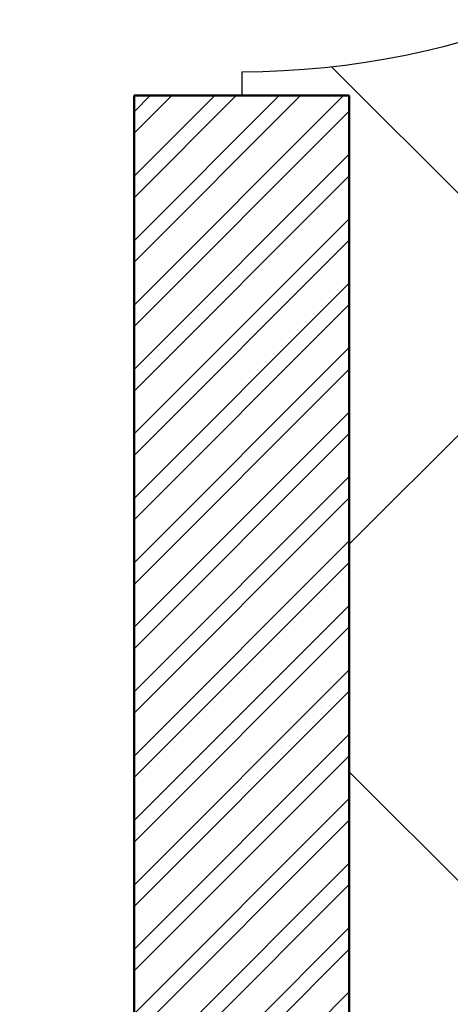
# Model space of a CAD drawing. Units: inches. Extents: x 3590 to 5167, y 65 to 1917.
# Tile 64 of 100: x 4919 to 4937, y 1681 to 1722. Entities that reach past the tile are written whole.
import ezdxf

# ---------------------------------------------------------------- set-up
doc = ezdxf.new("R2010")
doc.units = ezdxf.units.IN
for name, color, linetype, lineweight in [('A-DOOR', 3, 'Continuous', 25), ('A-FLOR-PATT', 8, 'Continuous', 13), ('A-WALL', 7, 'Continuous', 50), ('A-WALL-PATT', 251, 'Continuous', 13)]:
    doc.layers.add(name, color=color, linetype=linetype, lineweight=lineweight)

# ---------------------------------------------------------------- blocks, each defined once
blk = doc.blocks.new('D1')
for p, q in [((1, 0), (1, 34)), ((2, 0), (2, 33.985)), ((0, 0), (2, 0)), ((35, 0), (36, 0))]:
    blk.add_line(p, q)
at = {"ltscale": 0.5}
blk.add_arc((1, 0), 34, 0, 90, dxfattribs=at)

msp = doc.modelspace()

# ---------------------------------------------------------------- hatches: boundary and pattern name
at = {"layer": 'A-FLOR-PATT', "transparency": 33554687}
h = msp.add_hatch(dxfattribs=at)
h.set_pattern_fill('AR-HBONE', color=256, scale=0.2)
h.set_pattern_definition([(45, (-588.972, 0), (0, 28.73682), [60.96, -20.32]), (135, (-574.604, 14.368), (3e-15, 28.73682), [60.96, -20.32])])
h.paths.add_polyline_path([(5071.274, 1796.999), (4933.274, 1796.999), (4933.274, 1753.999), (4962.774, 1753.999, -0.414214), (4928.774, 1719.999), (4933.274, 1718.999), (4933.274, 1334.999), (5071.274, 1334.999)])
h.paths.add_polyline_path([(4951.78, 1521.077), (4951.715, 1521.04), (4951.563, 1520.895)], flags=16)
h.paths.add_polyline_path([(4952.267, 1521.376), (4952.198, 1521.371), (4952.198, 1521.356)], flags=0)
h.paths.add_polyline_path([(4967.051, 1529.728), (4965.231, 1528.694), (4963.411, 1527.714), (4961.756, 1526.851), (4963.589, 1527.449), (4964.036, 1527.478), (4962.975, 1527.249), (4961.76, 1526.852), (4959.792, 1525.834), (4958.005, 1524.895), (4956.24, 1523.93), (4954.504, 1522.919), (4954.129, 1522.682), (4953.361, 1521.997), (4953.366, 1521.998), (4953.605, 1522.064), (4955.106, 1522.761), (4956.921, 1523.434), (4958.678, 1523.915), (4960.358, 1524.2), (4961.945, 1524.286), (4964.171, 1524.108), (4965.958, 1523.309), (4963.863, 1522.976), (4965.187, 1522.499), (4963.366, 1522.497), (4961.545, 1522.487), (4959.764, 1522.461), (4958.304, 1522.419), (4957.974, 1522.388), (4956.307, 1522.232), (4954.718, 1522.071), (4953.251, 1521.899), (4953.525, 1521.623), (4954.331, 1521.379), (4956.243, 1521.23), (4958.039, 1520.93), (4959.684, 1520.483), (4961.16, 1519.896), (4963.107, 1518.8), (4964.393, 1517.325), (4962.973, 1517.726), (4964.558, 1516.661), (4965.407, 1515.708), (4963.507, 1516.322), (4961.68, 1517.005), (4959.935, 1517.745), (4958.282, 1518.528), (4956.732, 1519.343), (4955.295, 1520.175), (4954.672, 1520.572), (4954.513, 1520.627), (4955.658, 1519.318), (4956.703, 1517.982), (4957.644, 1516.647), (4958.485, 1515.334), (4959.55, 1513.524), (4960.438, 1511.769), (4958.841, 1513.62), (4957.452, 1515.325), (4955.819, 1517.459), (4956.665, 1515.448), (4957.111, 1513.923), (4957.447, 1511.714), (4957.076, 1509.793), (4956.538, 1511.11), (4955.992, 1512.569), (4955.444, 1514.125), (4954.898, 1515.735), (4954.357, 1517.356), (4953.824, 1518.943), (4953.305, 1520.452), (4953.065, 1521.116), (4952.971, 1521.146), (4952.949, 1521.086), (4952.73, 1520.199), (4953.37, 1518.024), (4953.757, 1516.373), (4954.051, 1514.765), (4954.264, 1513.221), (4954.471, 1511.131), (4954.497, 1510.402), (4954.409, 1511.76), (4954.264, 1513.221), (4954.051, 1514.765), (4953.757, 1516.373), (4953.37, 1518.024), (4952.877, 1519.698), (4952.716, 1520.141), (4952.533, 1519.059), (4952.374, 1517.789), (4952.219, 1516.312), (4952.046, 1514.6), (4951.833, 1512.626), (4951.557, 1510.363), (4951.203, 1512.168), (4950.852, 1514.339), (4950.985, 1516.376), (4951.66, 1518.286), (4952.593, 1520.481), (4952.357, 1521.13), (4951.855, 1520.328), (4950.839, 1518.908), (4949.777, 1517.587), (4948.916, 1516.617), (4948.111, 1515.256), (4947.089, 1513.554), (4945.889, 1511.615), (4946.326, 1513.402), (4946.562, 1514.249), (4945.528, 1513.327), (4944.581, 1512.531), (4946.018, 1514.508), (4947.204, 1516.048), (4947.893, 1517.313), (4949.307, 1518.764), (4950.414, 1519.767), (4950.451, 1519.806), (4952.267, 1521.376), (4951.645, 1521.493), (4950.404, 1521.18), (4948.044, 1520.359), (4946.119, 1519.452), (4944.572, 1518.475), (4943.35, 1517.443), (4941.997, 1515.92), (4941.661, 1515.275), (4942.813, 1516.99), (4944.572, 1518.475), (4946.119, 1519.452), (4948.044, 1520.359), (4950.404, 1521.18), (4951.645, 1521.493), (4949.647, 1521.868), (4948.6, 1521.756), (4947.126, 1521.57), (4945.42, 1521.348), (4943.45, 1521.105), (4941.183, 1520.856), (4942.86, 1521.613), (4943.873, 1522.03), (4942.952, 1521.909), (4941.41, 1521.485), (4939.543, 1520.67), (4938.968, 1520.226), (4940.733, 1521.299), (4942.952, 1521.909), (4943.702, 1522.008), (4945.894, 1522.7), (4947.565, 1522.714), (4948.921, 1522.566), (4951.131, 1522.183), (4950.971, 1522.297), (4948.129, 1523.006), (4946.035, 1523.707), (4944.232, 1524.521), (4942.707, 1525.461), (4941.444, 1526.537), (4940.43, 1527.761), (4939.649, 1529.143), (4941.421, 1528.122), (4943.147, 1527.132), (4944.841, 1526.175), (4946.514, 1525.25), (4948.179, 1524.359), (4948.365, 1524.263), (4946.475, 1526.045), (4945.181, 1527.54), (4944.19, 1529.033), (4943.496, 1530.54), (4943.278, 1531.36), (4942.498, 1531.919), (4943.114, 1531.762), (4942.959, 1533.659), (4944.14, 1531.989), (4944.612, 1531.323), (4946.202, 1530.463), (4947.486, 1529.509), (4948.79, 1528.226), (4950.368, 1526.237), (4949.485, 1528.155), (4948.851, 1530.123), (4948.491, 1532.041), (4948.381, 1533.918), (4948.501, 1535.76), (4948.827, 1537.573), (4949.418, 1535.565), (4949.957, 1533.569), (4950.464, 1531.586), (4950.961, 1529.617), (4951.391, 1527.954), (4951.724, 1530.687), (4952.201, 1532.58), (4952.889, 1534.33), (4953.77, 1535.951), (4954.827, 1537.46), (4954.521, 1535.39), (4954.273, 1533.937), (4955.58, 1535.663), (4956.748, 1536.739), (4956.159, 1534.78), (4955.589, 1532.873), (4955.043, 1531.006), (4954.525, 1529.166), (4954.038, 1527.341), (4953.638, 1525.733), (4953.611, 1525.586), (4953.398, 1524.166), (4953.382, 1524.009), (4954.07, 1525.476), (4954.912, 1527.022), (4956.136, 1528.894), (4957.847, 1530.577), (4959.376, 1531.54), (4958.256, 1530.104), (4957.143, 1528.663), (4956.066, 1527.243), (4955.056, 1525.871), (4954.141, 1524.571), (4953.352, 1523.372), (4953.311, 1523.303), (4953.273, 1522.925), (4953.261, 1522.382), (4954.103, 1523.373), (4954.63, 1524.284), (4955.961, 1526.358), (4957.23, 1528.13), (4958.421, 1529.609), (4960.037, 1531.368), (4961.374, 1532.375), (4962.101, 1532.77), (4961.07, 1531.061), (4959.987, 1529.438), (4958.869, 1527.908), (4958.15, 1527.007), (4959.803, 1528.003), (4961.589, 1528.793), (4963.391, 1529.328), (4965.211, 1529.632)], flags=16)
h.paths.add_polyline_path([(4962.944, 1523.182), (4961.107, 1523.422), (4960.392, 1523.362), (4962.35, 1523.331)], flags=0)
h.paths.add_polyline_path([(5049.541, 1584.551), (5049.476, 1584.515), (5049.325, 1584.37)], flags=16)
h.paths.add_polyline_path([(5050.028, 1584.851), (5049.959, 1584.845), (5049.959, 1584.83)], flags=0)
h.paths.add_polyline_path([(5042.333, 1581.949), (5043.88, 1582.926), (5045.806, 1583.833), (5048.165, 1584.654), (5049.406, 1584.967), (5047.408, 1585.342), (5046.361, 1585.231), (5044.888, 1585.044), (5043.181, 1584.822), (5041.211, 1584.579), (5038.944, 1584.33), (5040.622, 1585.087), (5041.634, 1585.504), (5040.713, 1585.383), (5039.171, 1584.959), (5037.304, 1584.144), (5036.729, 1583.7), (5038.494, 1584.773), (5040.713, 1585.383), (5041.463, 1585.482), (5043.655, 1586.174), (5045.326, 1586.188), (5046.682, 1586.04), (5048.893, 1585.657), (5048.732, 1585.771), (5045.891, 1586.48), (5043.796, 1587.181), (5041.994, 1587.996), (5040.468, 1588.935), (5039.205, 1590.011), (5038.191, 1591.235), (5037.41, 1592.617), (5039.182, 1591.596), (5040.909, 1590.607), (5042.602, 1589.649), (5044.275, 1588.724), (5045.94, 1587.833), (5046.126, 1587.738), (5044.237, 1589.519), (5042.942, 1591.015), (5041.952, 1592.508), (5041.257, 1594.014), (5041.039, 1594.834), (5040.26, 1595.393), (5040.875, 1595.237), (5040.721, 1597.133), (5041.901, 1595.463), (5042.373, 1594.798), (5043.963, 1593.938), (5045.247, 1592.983), (5046.552, 1591.701), (5048.129, 1589.712), (5047.247, 1591.63), (5046.613, 1593.597), (5046.252, 1595.515), (5046.142, 1597.392), (5046.262, 1599.234), (5046.588, 1601.047), (5047.179, 1599.039), (5047.718, 1597.043), (5048.225, 1595.06), (5048.722, 1593.091), (5049.152, 1591.429), (5049.485, 1594.161), (5049.962, 1596.054), (5050.65, 1597.804), (5051.532, 1599.425), (5052.589, 1600.934), (5052.283, 1598.864), (5052.034, 1597.411), (5053.341, 1599.137), (5054.509, 1600.213), (5053.92, 1598.254), (5053.35, 1596.348), (5052.805, 1594.48), (5052.286, 1592.64), (5051.799, 1590.815), (5051.4, 1589.207), (5051.373, 1589.06), (5051.159, 1587.64), (5051.143, 1587.483), (5051.831, 1588.95), (5052.673, 1590.496), (5053.898, 1592.368), (5055.608, 1594.051), (5057.137, 1595.014), (5056.017, 1593.578), (5054.904, 1592.137), (5053.828, 1590.717), (5052.817, 1589.345), (5051.902, 1588.046), (5051.113, 1586.846), (5051.072, 1586.777), (5051.034, 1586.399), (5051.022, 1585.856), (5051.864, 1586.847), (5052.391, 1587.758), (5053.723, 1589.832), (5054.991, 1591.604), (5056.182, 1593.083), (5057.798, 1594.842), (5059.135, 1595.849), (5059.863, 1596.244), (5058.831, 1594.535), (5057.749, 1592.912), (5056.63, 1591.382), (5055.912, 1590.482), (5057.564, 1591.477), (5059.35, 1592.267), (5061.152, 1592.802), (5062.972, 1593.106), (5064.812, 1593.203), (5062.992, 1592.169), (5061.172, 1591.188), (5059.518, 1590.325), (5061.35, 1590.924), (5061.797, 1590.952), (5060.737, 1590.723), (5059.521, 1590.326), (5057.553, 1589.308), (5055.766, 1588.369), (5054.002, 1587.404), (5052.265, 1586.393), (5051.891, 1586.156), (5051.122, 1585.471), (5051.127, 1585.472), (5051.366, 1585.538), (5052.867, 1586.235), (5054.682, 1586.908), (5056.439, 1587.389), (5058.12, 1587.675), (5059.706, 1587.76), (5061.933, 1587.583), (5063.719, 1586.783), (5061.624, 1586.45), (5062.949, 1585.973), (5061.127, 1585.971), (5059.307, 1585.961), (5057.525, 1585.935), (5056.065, 1585.893), (5055.735, 1585.862), (5054.068, 1585.707), (5052.479, 1585.546), (5051.012, 1585.373), (5051.286, 1585.097), (5052.092, 1584.853), (5054.004, 1584.704), (5055.8, 1584.404), (5057.446, 1583.958), (5058.921, 1583.37), (5060.868, 1582.274), (5062.154, 1580.799), (5060.734, 1581.2), (5062.32, 1580.135), (5063.168, 1579.182), (5061.269, 1579.796), (5059.441, 1580.479), (5057.696, 1581.219), (5056.043, 1582.003), (5054.493, 1582.817), (5053.057, 1583.649), (5052.433, 1584.047), (5052.274, 1584.101), (5053.42, 1582.793), (5054.464, 1581.457), (5055.405, 1580.121), (5056.247, 1578.809), (5057.311, 1576.998), (5058.199, 1575.244), (5056.602, 1577.094), (5055.213, 1578.799), (5053.58, 1580.933), (5054.427, 1578.922), (5054.872, 1577.397), (5055.208, 1575.189), (5054.838, 1573.267), (5054.299, 1574.584), (5053.754, 1576.043), (5053.206, 1577.599), (5052.659, 1579.209), (5052.118, 1580.83), (5051.585, 1582.417), (5051.066, 1583.927), (5050.826, 1584.59), (5050.733, 1584.62), (5050.711, 1584.561), (5050.491, 1583.673), (5051.131, 1581.498), (5051.518, 1579.847), (5051.813, 1578.24), (5052.026, 1576.695), (5052.233, 1574.605), (5052.258, 1573.876), (5052.17, 1575.234), (5052.026, 1576.695), (5051.813, 1578.24), (5051.518, 1579.847), (5051.131, 1581.498), (5050.638, 1583.172), (5050.477, 1583.615), (5050.294, 1582.533), (5050.136, 1581.263), (5049.981, 1579.786), (5049.807, 1578.074), (5049.594, 1576.1), (5049.318, 1573.837), (5048.965, 1575.642), (5048.613, 1577.813), (5048.747, 1579.85), (5049.421, 1581.76), (5050.354, 1583.955), (5050.118, 1584.604), (5049.616, 1583.802), (5048.6, 1582.382), (5047.538, 1581.061), (5046.677, 1580.091), (5045.872, 1578.73), (5044.85, 1577.028), (5043.651, 1575.089), (5044.087, 1576.877), (5044.324, 1577.723), (5043.289, 1576.801), (5042.342, 1576.005), (5043.779, 1577.982), (5044.966, 1579.522), (5045.655, 1580.787), (5047.068, 1582.239), (5048.175, 1583.241), (5048.213, 1583.28), (5050.028, 1584.851), (5049.406, 1584.967), (5048.165, 1584.654), (5045.806, 1583.833), (5043.88, 1582.926), (5042.333, 1581.949), (5041.111, 1580.917), (5039.758, 1579.394), (5039.423, 1578.749), (5040.575, 1580.464)], flags=16)
h.paths.add_polyline_path([(4954.799, 1533.12), (4954.262, 1532.079), (4953.831, 1530.935), (4953.505, 1529.636), (4953.283, 1528.133), (4953.167, 1526.376), (4953.156, 1524.315), (4953.277, 1521.236), (4952.802, 1521.842), (4951.557, 1521.998), (4950.976, 1521.961), (4952.661, 1521.941), (4952.802, 1521.842), (4953.152, 1523.593), (4953.167, 1526.376), (4953.283, 1528.133), (4953.609, 1530.346), (4954.456, 1532.592)], flags=0)
h.paths.add_polyline_path([(5050.563, 1585.316), (5049.318, 1585.472), (5048.737, 1585.435), (5050.422, 1585.415), (5050.563, 1585.316), (5050.914, 1587.067), (5050.928, 1589.851), (5051.045, 1591.607), (5051.371, 1593.82), (5052.217, 1596.066), (5052.56, 1596.594), (5052.024, 1595.554), (5051.592, 1594.409), (5051.266, 1593.11), (5051.045, 1591.607), (5050.928, 1589.851), (5050.918, 1587.789), (5051.038, 1584.71)], flags=0)
h.paths.add_polyline_path([(5058.153, 1586.836), (5060.111, 1586.805), (5060.705, 1586.656), (5058.868, 1586.896)], flags=0)
h.paths.add_polyline_path([(5049.541, 1430.936), (5049.476, 1430.9), (5049.325, 1430.755)], flags=16)
h.paths.add_polyline_path([(5050.028, 1431.236), (5049.959, 1431.231), (5049.959, 1431.215)], flags=0)
h.paths.add_polyline_path([(5046.588, 1447.432), (5047.179, 1445.425), (5047.718, 1443.429), (5048.225, 1441.446), (5048.722, 1439.476), (5049.152, 1437.814), (5049.485, 1440.546), (5049.962, 1442.439), (5050.65, 1444.189), (5051.532, 1445.811), (5052.589, 1447.319), (5052.283, 1445.249), (5052.034, 1443.796), (5053.341, 1445.522), (5054.509, 1446.598), (5053.92, 1444.64), (5053.35, 1442.733), (5052.805, 1440.865), (5052.286, 1439.025), (5051.799, 1437.201), (5051.4, 1435.592), (5051.373, 1435.445), (5051.159, 1434.025), (5051.143, 1433.868), (5051.831, 1435.335), (5052.673, 1436.881), (5053.898, 1438.753), (5055.608, 1440.436), (5057.137, 1441.4), (5056.017, 1439.963), (5054.904, 1438.522), (5053.828, 1437.102), (5052.817, 1435.73), (5051.902, 1434.431), (5051.113, 1433.231), (5051.072, 1433.162), (5051.034, 1432.784), (5051.022, 1432.242), (5051.864, 1433.232), (5052.391, 1434.143), (5053.723, 1436.217), (5054.991, 1437.989), (5056.182, 1439.468), (5057.798, 1441.227), (5059.135, 1442.235), (5059.863, 1442.629), (5058.831, 1440.921), (5057.749, 1439.298), (5056.63, 1437.767), (5055.912, 1436.867), (5057.564, 1437.863), (5059.35, 1438.652), (5061.152, 1439.187), (5062.972, 1439.491), (5064.812, 1439.588), (5062.992, 1438.554), (5061.172, 1437.573), (5059.518, 1436.71), (5061.35, 1437.309), (5061.797, 1437.337), (5060.737, 1437.108), (5059.521, 1436.711), (5057.553, 1435.693), (5055.766, 1434.754), (5054.002, 1433.789), (5052.265, 1432.778), (5051.891, 1432.541), (5051.122, 1431.856), (5051.127, 1431.857), (5051.366, 1431.923), (5052.867, 1432.62), (5054.682, 1433.293), (5056.439, 1433.775), (5058.12, 1434.06), (5059.706, 1434.145), (5061.933, 1433.968), (5063.719, 1433.168), (5061.624, 1432.835), (5062.949, 1432.358), (5061.127, 1432.357), (5059.307, 1432.346), (5057.525, 1432.32), (5056.065, 1432.278), (5055.735, 1432.248), (5054.068, 1432.092), (5052.479, 1431.931), (5051.012, 1431.759), (5051.286, 1431.482), (5052.092, 1431.238), (5054.004, 1431.089), (5055.8, 1430.789), (5057.446, 1430.343), (5058.921, 1429.755), (5060.868, 1428.66), (5062.154, 1427.185), (5060.734, 1427.585), (5062.32, 1426.52), (5063.168, 1425.567), (5061.269, 1426.181), (5059.441, 1426.865), (5057.696, 1427.604), (5056.043, 1428.388), (5054.493, 1429.202), (5053.057, 1430.034), (5052.433, 1430.432), (5052.274, 1430.487), (5053.42, 1429.178), (5054.464, 1427.842), (5055.405, 1426.506), (5056.247, 1425.194), (5057.311, 1423.383), (5058.199, 1421.629), (5056.602, 1423.479), (5055.213, 1425.184), (5053.58, 1427.318), (5054.427, 1425.307), (5054.872, 1423.782), (5055.208, 1421.574), (5054.838, 1419.652), (5054.299, 1420.97), (5053.754, 1422.428), (5053.206, 1423.984), (5052.659, 1425.595), (5052.118, 1427.215), (5051.585, 1428.802), (5051.066, 1430.312), (5050.826, 1430.975), (5050.733, 1431.005), (5050.711, 1430.946), (5050.491, 1430.058), (5051.131, 1427.883), (5051.518, 1426.232), (5051.813, 1424.625), (5052.026, 1423.081), (5052.233, 1420.991), (5052.258, 1420.261), (5052.17, 1421.619), (5052.026, 1423.081), (5051.813, 1424.625), (5051.518, 1426.232), (5051.131, 1427.883), (5050.638, 1429.558), (5050.477, 1430.001), (5050.294, 1428.918), (5050.136, 1427.648), (5049.981, 1426.171), (5049.807, 1424.459), (5049.594, 1422.485), (5049.318, 1420.222), (5048.965, 1422.028), (5048.613, 1424.199), (5048.747, 1426.235), (5049.421, 1428.146), (5050.354, 1430.34), (5050.118, 1430.989), (5049.616, 1430.187), (5048.6, 1428.768), (5047.538, 1427.446), (5046.677, 1426.477), (5045.872, 1425.116), (5044.85, 1423.413), (5043.651, 1421.474), (5044.087, 1423.262), (5044.324, 1424.109), (5043.289, 1423.186), (5042.342, 1422.391), (5043.779, 1424.368), (5044.966, 1425.907), (5045.655, 1427.173), (5047.068, 1428.624), (5048.175, 1429.627), (5048.213, 1429.666), (5050.028, 1431.236), (5049.406, 1431.353), (5048.165, 1431.039), (5045.806, 1430.218), (5043.88, 1429.311), (5042.333, 1428.334), (5041.111, 1427.302), (5039.758, 1425.779), (5039.423, 1425.134), (5040.575, 1426.849), (5042.333, 1428.334), (5043.88, 1429.311), (5045.806, 1430.218), (5048.165, 1431.039), (5049.406, 1431.353), (5047.408, 1431.727), (5046.361, 1431.616), (5044.888, 1431.429), (5043.181, 1431.207), (5041.211, 1430.964), (5038.944, 1430.715), (5040.622, 1431.472), (5041.634, 1431.89), (5040.713, 1431.769), (5039.171, 1431.345), (5037.304, 1430.53), (5036.729, 1430.085), (5038.494, 1431.158), (5040.713, 1431.769), (5041.463, 1431.867), (5043.655, 1432.559), (5045.326, 1432.573), (5046.682, 1432.425), (5048.893, 1432.042), (5048.732, 1432.156), (5045.891, 1432.865), (5043.796, 1433.566), (5041.994, 1434.381), (5040.468, 1435.321), (5039.205, 1436.396), (5038.191, 1437.62), (5037.41, 1439.002), (5039.182, 1437.982), (5040.909, 1436.992), (5042.602, 1436.034), (5044.275, 1435.109), (5045.94, 1434.218), (5046.126, 1434.123), (5044.237, 1435.904), (5042.942, 1437.4), (5041.952, 1438.893), (5041.257, 1440.399), (5041.039, 1441.219), (5040.26, 1441.778), (5040.875, 1441.622), (5040.721, 1443.518), (5041.901, 1441.848), (5042.373, 1441.183), (5043.963, 1440.323), (5045.247, 1439.369), (5046.552, 1438.086), (5048.129, 1436.097), (5047.247, 1438.015), (5046.613, 1439.982), (5046.252, 1441.901), (5046.142, 1443.778), (5046.262, 1445.619)], flags=16)
h.paths.add_polyline_path([(5052.382, 1444.255), (5051.623, 1442.78), (5052.024, 1441.939), (5052.56, 1442.98)], flags=0)
h.paths.add_polyline_path([(5050.563, 1431.701), (5049.318, 1431.857), (5048.737, 1431.821), (5050.422, 1431.8)], flags=0)
h.paths.add_polyline_path([(5058.153, 1433.221), (5060.111, 1433.19), (5060.705, 1433.041), (5058.868, 1433.281)], flags=0)
h.paths.add_polyline_path([(5049.541, 1352.285), (5049.476, 1352.249), (5049.325, 1352.104)], flags=16)
h.paths.add_polyline_path([(5050.028, 1352.585), (5049.959, 1352.58), (5049.959, 1352.564)], flags=0)
h.paths.add_polyline_path([(5046.588, 1368.781), (5047.179, 1366.774), (5047.718, 1364.778), (5048.225, 1362.795), (5048.722, 1360.825), (5049.152, 1359.163), (5049.485, 1361.896), (5049.962, 1363.789), (5050.65, 1365.538), (5051.532, 1367.16), (5052.589, 1368.669), (5052.283, 1366.598), (5052.034, 1365.145), (5053.341, 1366.871), (5054.509, 1367.947), (5053.92, 1365.989), (5053.35, 1364.082), (5052.805, 1362.214), (5052.286, 1360.374), (5051.799, 1358.55), (5051.4, 1356.942), (5051.373, 1356.794), (5051.159, 1355.374), (5051.143, 1355.218), (5051.831, 1356.684), (5052.673, 1358.23), (5053.898, 1360.102), (5055.608, 1361.786), (5057.137, 1362.749), (5056.017, 1361.313), (5054.904, 1359.872), (5053.828, 1358.452), (5052.817, 1357.079), (5051.902, 1355.78), (5051.113, 1354.581), (5051.072, 1354.512), (5051.034, 1354.133), (5051.022, 1353.591), (5051.864, 1354.581), (5052.391, 1355.492), (5053.723, 1357.566), (5054.991, 1359.338), (5056.182, 1360.817), (5057.798, 1362.577), (5059.135, 1363.584), (5059.863, 1363.979), (5058.831, 1362.27), (5057.749, 1360.647), (5056.63, 1359.117), (5055.912, 1358.216), (5057.564, 1359.212), (5059.35, 1360.001), (5061.152, 1360.536), (5062.972, 1360.841), (5064.812, 1360.937), (5062.992, 1359.903), (5061.172, 1358.923), (5059.518, 1358.059), (5061.35, 1358.658), (5061.797, 1358.687), (5060.737, 1358.458), (5059.521, 1358.061), (5057.553, 1357.043), (5055.766, 1356.103), (5054.002, 1355.138), (5052.265, 1354.127), (5051.891, 1353.89), (5051.122, 1353.206), (5051.127, 1353.206), (5051.366, 1353.272), (5052.867, 1353.969), (5054.682, 1354.643), (5056.439, 1355.124), (5058.12, 1355.409), (5059.706, 1355.495), (5061.933, 1355.317), (5063.719, 1354.518), (5061.624, 1354.184), (5062.949, 1353.708), (5061.127, 1353.706), (5059.307, 1353.695), (5057.525, 1353.669), (5056.065, 1353.627), (5055.735, 1353.597), (5054.068, 1353.441), (5052.479, 1353.28), (5051.012, 1353.108), (5051.286, 1352.831), (5052.092, 1352.587), (5054.004, 1352.439), (5055.8, 1352.138), (5057.446, 1351.692), (5058.921, 1351.104), (5060.868, 1350.009), (5062.154, 1348.534), (5060.734, 1348.935), (5062.32, 1347.869), (5063.168, 1346.916), (5061.269, 1347.53), (5059.441, 1348.214), (5057.696, 1348.954), (5056.043, 1349.737), (5054.493, 1350.551), (5053.057, 1351.383), (5052.433, 1351.781), (5052.274, 1351.836), (5053.42, 1350.527), (5054.464, 1349.191), (5055.405, 1347.855), (5056.247, 1346.543), (5057.311, 1344.733), (5058.199, 1342.978), (5056.602, 1344.828), (5055.213, 1346.534), (5053.58, 1348.667), (5054.427, 1346.656), (5054.872, 1345.132), (5055.208, 1342.923), (5054.838, 1341.002), (5054.299, 1342.319), (5053.754, 1343.778), (5053.206, 1345.334), (5052.659, 1346.944), (5052.118, 1348.564), (5051.585, 1350.151), (5051.066, 1351.661), (5050.826, 1352.324), (5050.733, 1352.355), (5050.711, 1352.295), (5050.491, 1351.408), (5051.131, 1349.232), (5051.518, 1347.581), (5051.813, 1345.974), (5052.026, 1344.43), (5052.233, 1342.34), (5052.258, 1341.61), (5052.17, 1342.969), (5052.026, 1344.43), (5051.813, 1345.974), (5051.518, 1347.581), (5051.131, 1349.232), (5050.638, 1350.907), (5050.477, 1351.35), (5050.294, 1350.267), (5050.136, 1348.997), (5049.981, 1347.52), (5049.807, 1345.809), (5049.594, 1343.835), (5049.318, 1341.571), (5048.965, 1343.377), (5048.613, 1345.548), (5048.747, 1347.585), (5049.421, 1349.495), (5050.354, 1351.689), (5050.118, 1352.339), (5049.616, 1351.536), (5048.6, 1350.117), (5047.538, 1348.795), (5046.677, 1347.826), (5045.872, 1346.465), (5044.85, 1344.763), (5043.651, 1342.824), (5044.087, 1344.611), (5044.324, 1345.458), (5043.289, 1344.535), (5042.342, 1343.74), (5043.779, 1345.717), (5044.966, 1347.256), (5045.655, 1348.522), (5047.068, 1349.973), (5048.175, 1350.976), (5048.213, 1351.015), (5050.028, 1352.585), (5049.406, 1352.702), (5048.165, 1352.388), (5045.806, 1351.567), (5043.88, 1350.661), (5042.333, 1349.683), (5041.111, 1348.651), (5039.758, 1347.128), (5039.423, 1346.483), (5040.575, 1348.198), (5042.333, 1349.683), (5043.88, 1350.661), (5045.806, 1351.567), (5048.165, 1352.388), (5049.406, 1352.702), (5047.408, 1353.076), (5046.361, 1352.965), (5044.888, 1352.779), (5043.181, 1352.556), (5041.211, 1352.313), (5038.944, 1352.065), (5040.622, 1352.821), (5041.634, 1353.239), (5040.713, 1353.118), (5039.171, 1352.694), (5037.304, 1351.879), (5036.729, 1351.434), (5038.494, 1352.508), (5040.713, 1353.118), (5041.463, 1353.216), (5043.655, 1353.909), (5045.326, 1353.923), (5046.682, 1353.774), (5048.893, 1353.391), (5048.732, 1353.506), (5045.891, 1354.214), (5043.796, 1354.915), (5041.994, 1355.73), (5040.468, 1356.67), (5039.205, 1357.746), (5038.191, 1358.969), (5037.41, 1360.352), (5039.182, 1359.331), (5040.909, 1358.341), (5042.602, 1357.383), (5044.275, 1356.458), (5045.94, 1355.567), (5046.126, 1355.472), (5044.237, 1357.253), (5042.942, 1358.749), (5041.952, 1360.242), (5041.257, 1361.748), (5041.039, 1362.568), (5040.26, 1363.128), (5040.875, 1362.971), (5040.721, 1364.867), (5041.901, 1363.197), (5042.373, 1362.532), (5043.963, 1361.672), (5045.247, 1360.718), (5046.552, 1359.435), (5048.129, 1357.446), (5047.247, 1359.364), (5046.613, 1361.331), (5046.252, 1363.25), (5046.142, 1365.127), (5046.262, 1366.969)], flags=16)
h.paths.add_polyline_path([(5052.382, 1365.604), (5051.623, 1364.129), (5052.024, 1363.288), (5052.56, 1364.329)], flags=0)
h.paths.add_polyline_path([(4951.78, 1698.041), (4951.715, 1698.005), (4951.563, 1697.859)], flags=16)
h.paths.add_polyline_path([(4952.267, 1698.341), (4952.198, 1698.335), (4952.198, 1698.32)], flags=0)
h.paths.add_polyline_path([(4957.076, 1686.757), (4956.538, 1688.074), (4955.992, 1689.533), (4955.444, 1691.089), (4954.898, 1692.699), (4954.357, 1694.32), (4953.824, 1695.907), (4953.305, 1697.417), (4953.065, 1698.08), (4952.971, 1698.11), (4952.949, 1698.051), (4952.73, 1697.163), (4953.37, 1694.988), (4953.757, 1693.337), (4954.051, 1691.729), (4954.264, 1690.185), (4954.471, 1688.095), (4954.497, 1687.366), (4954.409, 1688.724), (4954.264, 1690.185), (4954.051, 1691.729), (4953.757, 1693.337), (4953.37, 1694.988), (4952.877, 1696.662), (4952.716, 1697.105), (4952.533, 1696.023), (4952.374, 1694.753), (4952.219, 1693.276), (4952.046, 1691.564), (4951.833, 1689.59), (4951.557, 1687.327), (4951.203, 1689.132), (4950.852, 1691.303), (4950.985, 1693.34), (4951.66, 1695.25), (4952.593, 1697.445), (4952.357, 1698.094), (4951.855, 1697.292), (4950.839, 1695.872), (4949.777, 1694.551), (4948.916, 1693.581), (4948.111, 1692.22), (4947.089, 1690.518), (4945.889, 1688.579), (4946.326, 1690.366), (4946.562, 1691.213), (4945.528, 1690.291), (4944.581, 1689.495), (4946.018, 1691.472), (4947.204, 1693.012), (4947.893, 1694.277), (4949.307, 1695.729), (4950.414, 1696.731), (4950.451, 1696.77), (4952.267, 1698.341), (4951.645, 1698.457), (4950.404, 1698.144), (4948.044, 1697.323), (4946.119, 1696.416), (4944.572, 1695.439), (4943.35, 1694.407), (4941.997, 1692.884), (4941.661, 1692.239), (4942.813, 1693.954), (4944.572, 1695.439), (4946.119, 1696.416), (4948.044, 1697.323), (4950.404, 1698.144), (4951.645, 1698.457), (4949.647, 1698.832), (4948.6, 1698.72), (4947.126, 1698.534), (4945.42, 1698.312), (4943.45, 1698.069), (4941.183, 1697.82), (4942.86, 1698.577), (4943.873, 1698.994), (4942.952, 1698.873), (4941.41, 1698.449), (4939.543, 1697.634), (4938.968, 1697.19), (4940.733, 1698.263), (4942.952, 1698.873), (4943.702, 1698.972), (4945.894, 1699.664), (4947.565, 1699.678), (4948.921, 1699.53), (4951.131, 1699.147), (4950.971, 1699.261), (4948.129, 1699.97), (4946.035, 1700.671), (4944.232, 1701.486), (4942.707, 1702.425), (4941.444, 1703.501), (4940.43, 1704.725), (4939.649, 1706.107), (4941.421, 1705.086), (4943.147, 1704.097), (4944.841, 1703.139), (4946.514, 1702.214), (4948.179, 1701.323), (4948.365, 1701.227), (4946.475, 1703.009), (4945.181, 1704.505), (4944.19, 1705.997), (4943.496, 1707.504), (4943.278, 1708.324), (4942.498, 1708.883), (4943.114, 1708.727), (4942.959, 1710.623), (4944.14, 1708.953), (4944.612, 1708.287), (4946.202, 1707.428), (4947.486, 1706.473), (4948.79, 1705.191), (4950.368, 1703.202), (4949.485, 1705.12), (4948.851, 1707.087), (4948.491, 1709.005), (4948.381, 1710.882), (4948.501, 1712.724), (4948.827, 1714.537), (4949.418, 1712.529), (4949.957, 1710.533), (4950.464, 1708.55), (4950.961, 1706.581), (4951.391, 1704.919), (4951.724, 1707.651), (4952.201, 1709.544), (4952.889, 1711.294), (4953.77, 1712.915), (4954.827, 1714.424), (4954.521, 1712.354), (4954.273, 1710.901), (4955.58, 1712.627), (4956.748, 1713.703), (4956.159, 1711.744), (4955.589, 1709.837), (4955.043, 1707.97), (4954.525, 1706.13), (4954.038, 1704.305), (4953.638, 1702.697), (4953.611, 1702.55), (4953.398, 1701.13), (4953.382, 1700.973), (4954.07, 1702.44), (4954.912, 1703.986), (4956.136, 1705.858), (4957.847, 1707.541), (4959.376, 1708.504), (4958.256, 1707.068), (4957.143, 1705.627), (4956.066, 1704.207), (4955.056, 1702.835), (4954.141, 1701.536), (4953.352, 1700.336), (4953.311, 1700.267), (4953.273, 1699.889), (4953.261, 1699.346), (4954.103, 1700.337), (4954.63, 1701.248), (4955.961, 1703.322), (4957.23, 1705.094), (4958.421, 1706.573), (4960.037, 1708.332), (4961.374, 1709.339), (4962.101, 1709.734), (4961.07, 1708.025), (4959.987, 1706.402), (4958.869, 1704.872), (4958.15, 1703.972), (4959.803, 1704.967), (4961.589, 1705.757), (4963.391, 1706.292), (4965.211, 1706.596), (4967.051, 1706.692), (4965.231, 1705.659), (4963.411, 1704.678), (4961.756, 1703.815), (4963.589, 1704.413), (4964.036, 1704.442), (4962.975, 1704.213), (4961.76, 1703.816), (4959.792, 1702.798), (4958.005, 1701.859), (4956.24, 1700.894), (4954.504, 1699.883), (4954.129, 1699.646), (4953.361, 1698.961), (4953.366, 1698.962), (4953.605, 1699.028), (4955.106, 1699.725), (4956.921, 1700.398), (4958.678, 1700.879), (4960.358, 1701.164), (4961.945, 1701.25), (4964.171, 1701.073), (4965.958, 1700.273), (4963.863, 1699.94), (4965.187, 1699.463), (4963.366, 1699.461), (4961.545, 1699.451), (4959.764, 1699.425), (4958.304, 1699.383), (4957.974, 1699.352), (4956.307, 1699.197), (4954.718, 1699.036), (4953.251, 1698.863), (4953.525, 1698.587), (4954.331, 1698.343), (4956.243, 1698.194), (4958.039, 1697.894), (4959.684, 1697.447), (4961.16, 1696.86), (4963.107, 1695.764), (4964.393, 1694.289), (4962.973, 1694.69), (4964.558, 1693.625), (4965.407, 1692.672), (4963.507, 1693.286), (4961.68, 1693.969), (4959.935, 1694.709), (4958.282, 1695.492), (4956.732, 1696.307), (4955.295, 1697.139), (4954.672, 1697.536), (4954.513, 1697.591), (4955.658, 1696.282), (4956.703, 1694.946), (4957.644, 1693.611), (4958.485, 1692.298), (4959.55, 1690.488), (4960.438, 1688.733), (4958.841, 1690.584), (4957.452, 1692.289), (4955.819, 1694.423), (4956.665, 1692.412), (4957.111, 1690.887), (4957.447, 1688.678)], flags=16)
h.paths.add_polyline_path([(5050.563, 1353.05), (5049.318, 1353.207), (5048.737, 1353.17), (5050.422, 1353.15)], flags=0)
h.paths.add_polyline_path([(4951.78, 1351.486), (4951.715, 1351.45), (4951.563, 1351.305)], flags=16)
h.paths.add_polyline_path([(4952.267, 1351.786), (4952.198, 1351.78), (4952.198, 1351.765)], flags=0)
h.paths.add_polyline_path([(4954.827, 1367.869), (4954.521, 1365.799), (4954.273, 1364.346), (4955.58, 1366.072), (4956.748, 1367.148), (4956.159, 1365.19), (4955.589, 1363.283), (4955.043, 1361.415), (4954.525, 1359.575), (4954.038, 1357.751), (4953.638, 1356.142), (4953.611, 1355.995), (4953.398, 1354.575), (4953.382, 1354.418), (4954.07, 1355.885), (4954.912, 1357.431), (4956.136, 1359.303), (4957.847, 1360.986), (4959.376, 1361.95), (4958.256, 1360.513), (4957.143, 1359.072), (4956.066, 1357.652), (4955.056, 1356.28), (4954.141, 1354.981), (4953.352, 1353.781), (4953.311, 1353.712), (4953.273, 1353.334), (4953.261, 1352.792), (4954.103, 1353.782), (4954.63, 1354.693), (4955.961, 1356.767), (4957.23, 1358.539), (4958.421, 1360.018), (4960.037, 1361.777), (4961.374, 1362.785), (4962.101, 1363.179), (4961.07, 1361.471), (4959.987, 1359.848), (4958.869, 1358.317), (4958.15, 1357.417), (4959.803, 1358.413), (4961.589, 1359.202), (4963.391, 1359.737), (4965.211, 1360.041), (4967.051, 1360.138), (4965.231, 1359.104), (4963.411, 1358.123), (4961.756, 1357.26), (4963.589, 1357.859), (4964.036, 1357.887), (4962.975, 1357.658), (4961.76, 1357.261), (4959.792, 1356.243), (4958.005, 1355.304), (4956.24, 1354.339), (4954.504, 1353.328), (4954.129, 1353.091), (4953.361, 1352.406), (4953.366, 1352.407), (4953.605, 1352.473), (4955.106, 1353.17), (4956.921, 1353.843), (4958.678, 1354.325), (4960.358, 1354.61), (4961.945, 1354.695), (4964.171, 1354.518), (4965.958, 1353.718), (4963.863, 1353.385), (4965.187, 1352.908), (4963.366, 1352.907), (4961.545, 1352.896), (4959.764, 1352.87), (4958.304, 1352.828), (4957.974, 1352.798), (4956.307, 1352.642), (4954.718, 1352.481), (4953.251, 1352.309), (4953.525, 1352.032), (4954.331, 1351.788), (4956.243, 1351.639), (4958.039, 1351.339), (4959.684, 1350.893), (4961.16, 1350.305), (4963.107, 1349.21), (4964.393, 1347.735), (4962.973, 1348.135), (4964.558, 1347.07), (4965.407, 1346.117), (4963.507, 1346.731), (4961.68, 1347.414), (4959.935, 1348.154), (4958.282, 1348.938), (4956.732, 1349.752), (4955.295, 1350.584), (4954.672, 1350.982), (4954.513, 1351.036), (4955.658, 1349.728), (4956.703, 1348.392), (4957.644, 1347.056), (4958.485, 1345.744), (4959.55, 1343.933), (4960.438, 1342.179), (4958.841, 1344.029), (4957.452, 1345.734), (4955.819, 1347.868), (4956.665, 1345.857), (4957.111, 1344.332), (4957.447, 1342.124), (4957.076, 1340.202), (4956.538, 1341.52), (4955.992, 1342.978), (4955.444, 1344.534), (4954.898, 1346.145), (4954.357, 1347.765), (4953.824, 1349.352), (4953.305, 1350.862), (4953.065, 1351.525), (4952.971, 1351.555), (4952.949, 1351.496), (4952.73, 1350.608), (4953.37, 1348.433), (4953.757, 1346.782), (4954.051, 1345.175), (4954.264, 1343.631), (4954.471, 1341.541), (4954.497, 1340.811), (4954.409, 1342.169), (4954.264, 1343.631), (4954.051, 1345.175), (4953.757, 1346.782), (4953.37, 1348.433), (4952.877, 1350.108), (4952.716, 1350.551), (4952.533, 1349.468), (4952.374, 1348.198), (4952.219, 1346.721), (4952.046, 1345.009), (4951.833, 1343.035), (4951.557, 1340.772), (4951.203, 1342.578), (4950.852, 1344.749), (4950.985, 1346.785), (4951.66, 1348.696), (4952.593, 1350.89), (4952.357, 1351.539), (4951.855, 1350.737), (4950.839, 1349.318), (4949.777, 1347.996), (4948.916, 1347.027), (4948.111, 1345.665), (4947.089, 1343.963), (4945.889, 1342.024), (4946.326, 1343.812), (4946.562, 1344.659), (4945.528, 1343.736), (4944.581, 1342.941), (4946.018, 1344.918), (4947.204, 1346.457), (4947.893, 1347.723), (4949.307, 1349.174), (4950.414, 1350.177), (4950.451, 1350.216), (4952.267, 1351.786), (4951.645, 1351.903), (4950.404, 1351.589), (4948.044, 1350.768), (4946.119, 1349.861), (4944.572, 1348.884), (4943.35, 1347.852), (4941.997, 1346.329), (4941.661, 1345.684), (4942.813, 1347.399), (4944.572, 1348.884), (4946.119, 1349.861), (4948.044, 1350.768), (4950.404, 1351.589), (4951.645, 1351.903), (4949.647, 1352.277), (4948.6, 1352.166), (4947.126, 1351.979), (4945.42, 1351.757), (4943.45, 1351.514), (4941.183, 1351.265), (4942.86, 1352.022), (4943.873, 1352.44), (4942.952, 1352.319), (4941.41, 1351.895), (4939.543, 1351.08), (4938.968, 1350.635), (4940.733, 1351.708), (4942.952, 1352.319), (4943.702, 1352.417), (4945.894, 1353.109), (4947.565, 1353.123), (4948.921, 1352.975), (4951.131, 1352.592), (4950.971, 1352.706), (4948.129, 1353.415), (4946.035, 1354.116), (4944.232, 1354.931), (4942.707, 1355.871), (4941.444, 1356.946), (4940.43, 1358.17), (4939.649, 1359.552), (4941.421, 1358.532), (4943.147, 1357.542), (4944.841, 1356.584), (4946.514, 1355.659), (4948.179, 1354.768), (4948.365, 1354.673), (4946.475, 1356.454), (4945.181, 1357.95), (4944.19, 1359.443), (4943.496, 1360.949), (4943.278, 1361.769), (4942.498, 1362.328), (4943.114, 1362.172), (4942.959, 1364.068), (4944.14, 1362.398), (4944.612, 1361.733), (4946.202, 1360.873), (4947.486, 1359.919), (4948.79, 1358.636), (4950.368, 1356.647), (4949.485, 1358.565), (4948.851, 1360.532), (4948.491, 1362.451), (4948.381, 1364.328), (4948.501, 1366.169), (4948.827, 1367.982), (4949.418, 1365.975), (4949.957, 1363.979), (4950.464, 1361.995), (4950.961, 1360.026), (4951.391, 1358.364), (4951.724, 1361.096), (4952.201, 1362.989), (4952.889, 1364.739), (4953.77, 1366.361)], flags=16)
h.paths.add_polyline_path([(4954.799, 1363.53), (4954.262, 1362.489), (4953.831, 1361.344), (4953.505, 1360.045), (4953.283, 1358.543), (4953.167, 1356.786), (4953.156, 1354.724), (4953.277, 1351.646), (4952.802, 1352.251), (4951.557, 1352.407), (4950.976, 1352.371), (4952.661, 1352.35), (4952.802, 1352.251), (4953.152, 1354.002), (4953.167, 1356.786), (4953.283, 1358.543), (4953.609, 1360.755), (4954.456, 1363.001)], flags=0)
h.paths.add_polyline_path([(4952.802, 1698.806), (4951.557, 1698.962), (4950.976, 1698.925), (4952.661, 1698.905), (4952.802, 1698.806), (4953.152, 1700.557), (4953.167, 1703.34), (4953.283, 1705.097), (4953.609, 1707.31), (4954.456, 1709.556), (4954.799, 1710.084), (4954.262, 1709.043), (4953.831, 1707.899), (4953.505, 1706.6), (4953.283, 1705.097), (4953.167, 1703.34), (4953.156, 1701.279), (4953.277, 1698.2)], flags=0)
h.paths.add_polyline_path([(4962.944, 1700.146), (4961.107, 1700.386), (4960.392, 1700.326), (4962.35, 1700.295)], flags=0)
h.paths.add_polyline_path([(5058.153, 1354.57), (5060.111, 1354.539), (5060.705, 1354.391), (5058.868, 1354.631)], flags=0)
h.paths.add_polyline_path([(4962.944, 1353.591), (4961.107, 1353.831), (4960.392, 1353.771), (4962.35, 1353.74)], flags=0)
h.paths.add_polyline_path([(5049.541, 1778.72), (5049.476, 1778.684), (5049.325, 1778.539)], flags=16)
h.paths.add_polyline_path([(5050.028, 1779.02), (5049.959, 1779.014), (5049.959, 1778.999)], flags=0)
h.paths.add_polyline_path([(5052.258, 1768.045), (5052.17, 1769.403), (5052.026, 1770.864), (5051.813, 1772.409), (5051.518, 1774.016), (5051.131, 1775.667), (5050.638, 1777.341), (5050.477, 1777.784), (5050.294, 1776.702), (5050.136, 1775.432), (5049.981, 1773.955), (5049.807, 1772.243), (5049.594, 1770.269), (5049.318, 1768.006), (5048.965, 1769.811), (5048.613, 1771.982), (5048.747, 1774.019), (5049.421, 1775.929), (5050.354, 1778.124), (5050.118, 1778.773), (5049.616, 1777.971), (5048.6, 1776.551), (5047.538, 1775.23), (5046.677, 1774.26), (5045.872, 1772.899), (5044.85, 1771.197), (5043.651, 1769.258), (5044.087, 1771.046), (5044.324, 1771.892), (5043.289, 1770.97), (5042.342, 1770.174), (5043.779, 1772.151), (5044.966, 1773.691), (5045.655, 1774.956), (5047.068, 1776.408), (5048.175, 1777.41), (5048.213, 1777.449), (5050.028, 1779.02), (5049.406, 1779.136), (5048.165, 1778.823), (5045.806, 1778.002), (5043.88, 1777.095), (5042.333, 1776.118), (5041.111, 1775.086), (5039.758, 1773.563), (5039.423, 1772.918), (5040.575, 1774.633), (5042.333, 1776.118), (5043.88, 1777.095), (5045.806, 1778.002), (5048.165, 1778.823), (5049.406, 1779.136), (5047.408, 1779.511), (5046.361, 1779.4), (5044.888, 1779.213), (5043.181, 1778.991), (5041.211, 1778.748), (5038.944, 1778.499), (5040.622, 1779.256), (5041.634, 1779.673), (5040.713, 1779.552), (5039.171, 1779.128), (5037.304, 1778.313), (5036.729, 1777.869), (5038.494, 1778.942), (5040.713, 1779.552), (5041.463, 1779.651), (5043.655, 1780.343), (5045.326, 1780.357), (5046.682, 1780.209), (5048.893, 1779.826), (5048.732, 1779.94), (5045.891, 1780.649), (5043.796, 1781.35), (5041.994, 1782.165), (5040.468, 1783.104), (5039.205, 1784.18), (5038.191, 1785.404), (5037.41, 1786.786), (5039.182, 1785.765), (5040.909, 1784.776), (5042.602, 1783.818), (5044.275, 1782.893), (5045.94, 1782.002), (5046.126, 1781.907), (5044.237, 1783.688), (5042.942, 1785.184), (5041.952, 1786.677), (5041.257, 1788.183), (5041.039, 1789.003), (5040.26, 1789.562), (5040.875, 1789.406), (5040.721, 1791.302), (5041.901, 1789.632), (5042.373, 1788.967), (5043.963, 1788.107), (5045.247, 1787.152), (5046.552, 1785.87), (5048.129, 1783.881), (5047.247, 1785.799), (5046.613, 1787.766), (5046.252, 1789.684), (5046.142, 1791.561), (5046.262, 1793.403), (5046.588, 1795.216), (5047.179, 1793.208), (5047.718, 1791.213), (5048.225, 1789.229), (5048.722, 1787.26), (5049.152, 1785.598), (5049.485, 1788.33), (5049.962, 1790.223), (5050.65, 1791.973), (5051.532, 1793.594), (5052.589, 1795.103), (5052.283, 1793.033), (5052.034, 1791.58), (5053.341, 1793.306), (5054.509, 1794.382), (5053.92, 1792.423), (5053.35, 1790.517), (5052.805, 1788.649), (5052.286, 1786.809), (5051.799, 1784.984), (5051.4, 1783.376), (5051.373, 1783.229), (5051.159, 1781.809), (5051.143, 1781.652), (5051.831, 1783.119), (5052.673, 1784.665), (5053.898, 1786.537), (5055.608, 1788.22), (5057.137, 1789.183), (5056.017, 1787.747), (5054.904, 1786.306), (5053.828, 1784.886), (5052.817, 1783.514), (5051.902, 1782.215), (5051.113, 1781.015), (5051.072, 1780.946), (5051.034, 1780.568), (5051.022, 1780.025), (5051.864, 1781.016), (5052.391, 1781.927), (5053.723, 1784.001), (5054.991, 1785.773), (5056.182, 1787.252), (5057.798, 1789.011), (5059.135, 1790.018), (5059.863, 1790.413), (5058.831, 1788.704), (5057.749, 1787.081), (5056.63, 1785.551), (5055.912, 1784.651), (5057.564, 1785.646), (5059.35, 1786.436), (5061.152, 1786.971), (5062.972, 1787.275), (5064.812, 1787.372), (5062.992, 1786.338), (5061.172, 1785.357), (5059.518, 1784.494), (5061.35, 1785.093), (5061.797, 1785.121), (5060.737, 1784.892), (5059.521, 1784.495), (5057.553, 1783.477), (5055.766, 1782.538), (5054.002, 1781.573), (5052.265, 1780.562), (5051.891, 1780.325), (5051.122, 1779.64), (5051.127, 1779.641), (5051.366, 1779.707), (5052.867, 1780.404), (5054.682, 1781.077), (5056.439, 1781.558), (5058.12, 1781.844), (5059.706, 1781.929), (5061.933, 1781.752), (5063.719, 1780.952), (5061.624, 1780.619), (5062.949, 1780.142), (5061.127, 1780.14), (5059.307, 1780.13), (5057.525, 1780.104), (5056.065, 1780.062), (5055.735, 1780.031), (5054.068, 1779.876), (5052.479, 1779.715), (5051.012, 1779.542), (5051.286, 1779.266), (5052.092, 1779.022), (5054.004, 1778.873), (5055.8, 1778.573), (5057.446, 1778.127), (5058.921, 1777.539), (5060.868, 1776.443), (5062.154, 1774.968), (5060.734, 1775.369), (5062.32, 1774.304), (5063.168, 1773.351), (5061.269, 1773.965), (5059.441, 1774.648), (5057.696, 1775.388), (5056.043, 1776.172), (5054.493, 1776.986), (5053.057, 1777.818), (5052.433, 1778.216), (5052.274, 1778.27), (5053.42, 1776.962), (5054.464, 1775.626), (5055.405, 1774.29), (5056.247, 1772.978), (5057.311, 1771.167), (5058.199, 1769.413), (5056.602, 1771.263), (5055.213, 1772.968), (5053.58, 1775.102), (5054.427, 1773.091), (5054.872, 1771.566), (5055.208, 1769.358), (5054.838, 1767.436), (5054.299, 1768.753), (5053.754, 1770.212), (5053.206, 1771.768), (5052.659, 1773.378), (5052.118, 1774.999), (5051.585, 1776.586), (5051.066, 1778.096), (5050.826, 1778.759), (5050.733, 1778.789), (5050.711, 1778.73), (5050.491, 1777.842), (5051.131, 1775.667), (5051.518, 1774.016), (5051.813, 1772.409), (5052.026, 1770.864), (5052.233, 1768.774)], flags=16)
h.paths.add_polyline_path([(5050.563, 1779.485), (5049.318, 1779.641), (5048.737, 1779.604), (5050.422, 1779.584), (5050.563, 1779.485), (5050.914, 1781.236), (5050.928, 1784.02), (5051.045, 1785.776), (5051.371, 1787.989), (5052.217, 1790.235), (5052.56, 1790.763), (5052.024, 1789.723), (5051.592, 1788.578), (5051.266, 1787.279), (5051.045, 1785.776), (5050.928, 1784.02), (5050.918, 1781.958), (5051.038, 1778.879)], flags=0)
h.paths.add_polyline_path([(5058.153, 1781.005), (5060.111, 1780.974), (5060.705, 1780.825), (5058.868, 1781.065)], flags=0)
at = {"layer": 'A-WALL-PATT', "transparency": 33554687}
h = msp.add_hatch(dxfattribs=at)
h.set_pattern_fill('ANSI32', color=256, scale=0.2)
h.paths.add_polyline_path([(4684.274, 1805.999), (4591.274, 1805.999), (4591.274, 1796.999), (4639.274, 1796.999), (4639.274, 1790.999), (4648.274, 1790.999), (4648.274, 1796.999), (4684.274, 1796.999)])
h.paths.add_polyline_path([(4543.274, 1805.999), (4420.274, 1805.999), (4420.274, 1784.999), (4429.274, 1784.999), (4429.274, 1796.999), (4445.919, 1796.999), (4543.274, 1796.999)])
h.paths.add_polyline_path([(4828.274, 1805.999), (4744.274, 1805.999), (4744.274, 1796.999), (4828.274, 1796.999)])
h.paths.add_polyline_path([(4648.274, 1754.999), (4639.274, 1754.999), (4639.274, 1655.999), (4546.274, 1655.999), (4546.274, 1649.999), (4549.274, 1649.999), (4549.274, 1553.999), (4429.274, 1553.999), (4429.274, 1583.999), (4420.274, 1583.999), (4420.274, 1538.999), (4429.274, 1538.999), (4429.274, 1544.999), (4639.274, 1544.999), (4639.274, 1538.999), (4648.274, 1538.999), (4648.274, 1559.999), (4639.274, 1559.999), (4639.274, 1553.999), (4555.274, 1553.999), (4555.274, 1649.999), (4639.274, 1649.999), (4639.274, 1589.999), (4648.274, 1589.999)])
h.paths.add_polyline_path([(4516.274, 1655.999), (4429.274, 1655.999), (4429.274, 1736.999), (4420.274, 1736.999), (4420.274, 1619.999), (4429.274, 1619.999), (4429.274, 1649.999), (4516.274, 1649.999)], flags=17)
h.paths.add_polyline_path([(5080.274, 1805.999), (4888.274, 1805.999), (4888.274, 1796.999), (4924.274, 1796.999), (4924.274, 1754.999), (4933.274, 1754.999), (4933.274, 1796.999), (5071.274, 1796.999), (5071.274, 1334.999), (4933.274, 1334.999), (4933.274, 1565.999), (4924.274, 1565.999), (4924.274, 1334.999), (4898.774, 1334.999), (4898.774, 1325.999), (5080.274, 1325.999)])
h.paths.add_polyline_path([(4933.274, 1718.999), (4924.274, 1718.999), (4924.274, 1637.999), (4933.274, 1637.999)], flags=17)
h.paths.add_polyline_path([(4802.774, 1334.999), (4777.274, 1334.999), (4777.274, 1502.999), (4756.274, 1502.999), (4756.274, 1493.999), (4768.274, 1493.999), (4768.274, 1430.999), (4696.274, 1430.999), (4696.274, 1493.999), (4708.274, 1493.999), (4708.274, 1502.999), (4639.274, 1502.999), (4639.274, 1493.999), (4687.274, 1493.999), (4687.274, 1430.999), (4681.274, 1430.999), (4681.274, 1421.999), (4768.274, 1421.999), (4768.274, 1334.999), (4726.274, 1334.999), (4726.274, 1325.999), (4802.774, 1325.999)])
h.paths.add_polyline_path([(4690.274, 1334.999), (4648.274, 1334.999), (4648.274, 1352.867), (4648.274, 1421.999), (4651.274, 1421.999), (4651.274, 1430.999), (4639.274, 1430.999), (4639.274, 1334.999), (4633.274, 1334.999), (4633.274, 1325.999), (4690.274, 1325.999)])
h.paths.add_polyline_path([(4585.274, 1334.999), (4584.724, 1334.999), (4429.274, 1334.999), (4429.274, 1490.999), (4420.274, 1490.999), (4420.274, 1325.999), (4585.274, 1325.999)])

# ---------------------------------------------------------------- linework, layer by layer
at = {"layer": 'A-WALL'}
for p, q in [((4924.274, 1334.999), (4924.274, 1718.999)), ((4924.274, 1718.999), (4933.274, 1718.999)), ((4933.274, 1334.999), (4933.274, 1718.999))]:
    msp.add_line(p, q, dxfattribs=at)

# ---------------------------------------------------------------- block references
at = {"layer": 'A-DOOR', "rotation": 270}
msp.add_blockref('D1', (4928.774, 1754.999), dxfattribs=at)

doc.saveas('drawing.dxf')
